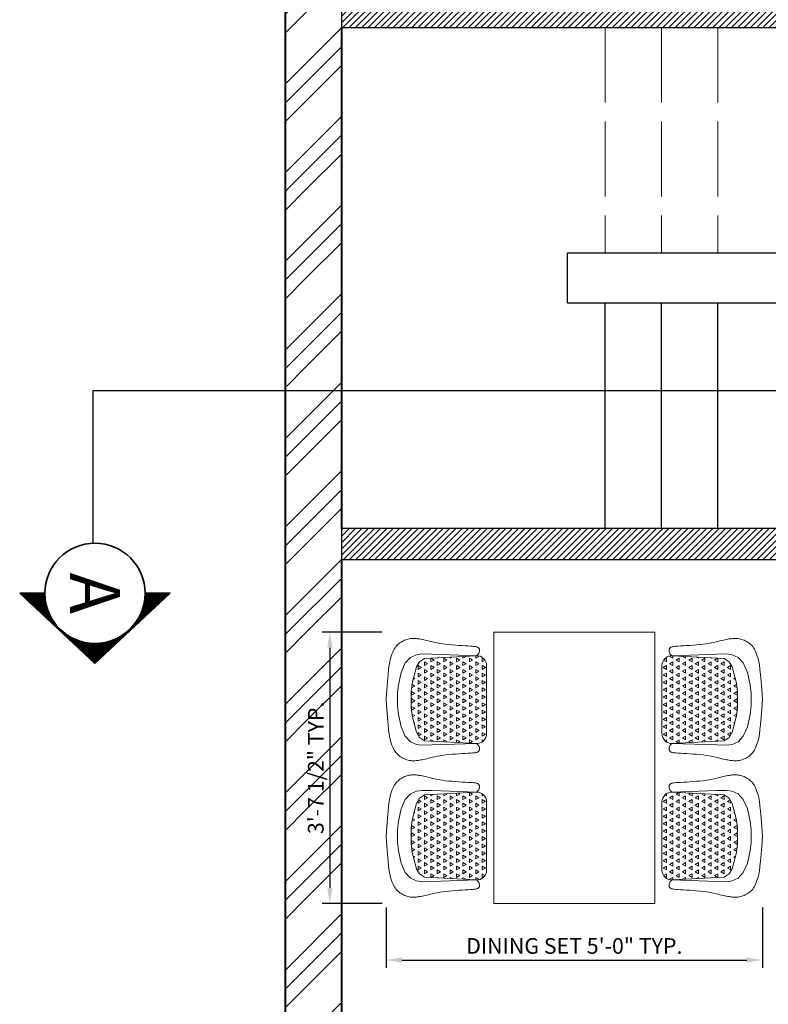
# Model space of a CAD drawing. Units: inches. Extents: x 2443635 to 2446153, y 1826255 to 1827341.
# Tile 2 of 16: x 2443665 to 2443784, y 1826991 to 1827149. Entities that reach past the tile are written whole.
import ezdxf
from ezdxf.enums import TextEntityAlignment as Align

# ---------------------------------------------------------------- set-up
doc = ezdxf.new("R2010")
doc.units = ezdxf.units.IN
doc.linetypes.add('ACAD_ISO02W100', pattern=[15, 12, -3])
for name, color, linetype, lineweight in [('A-ANNO-SYMB', 4, 'Continuous', 25), ('A-DIMS', 1, 'Continuous', 18), ('A-FURN', 6, 'Continuous', 18), ('A-SECT', 7, 'Continuous', 35), ('A-STAIR', 7, 'Continuous', 25), ('A-STAIR-OVHD', 7, 'ACAD_ISO02W100', 18), ('A-WALL-EXT', 7, 'Continuous', 40), ('A-WALL-INT', 9, 'Continuous', 30), ('A-WALL-PATT', 8, 'Continuous', 13)]:
    doc.layers.add(name, color=color, linetype=linetype, lineweight=lineweight)
doc.styles.add('KH-TRUC', font='txt', dxfattribs={"height": 200})
doc.styles.get("Standard").update_dxf_attribs({"font": 'arial.ttf'})
doc.dimstyles.new('ISO-25', dxfattribs={"dimtxt": 2.5, "dimasz": 2.5, "dimexe": 1.25, "dimexo": 0.625, "dimtad": 1, "dimlunit": 4, "dimtxsty": 'Standard', "dimcen": 2.5, "dimadec": 0, "dimazin": 0, "dimtfac": 1, "dimtmove": 0, "dimatfit": 3, "dimfxl": 1, "dimarcsym": 0})

# ---------------------------------------------------------------- blocks, each defined once
blk = doc.blocks.new('*X10')
at = {"color": 0}
for p, q in [((152.437, 136.074), (152.218, 136.074)), ((152.347, 136.232), (152.437, 136.074)), ((152.625, 135.749), (152.437, 135.425)), ((152.625, 135.749), (152.812, 135.425)), ((153, 136.399), (152.812, 136.074)), ((153.187, 136.074), (152.812, 136.074)), ((153, 136.399), (153.187, 136.074)), ((153.375, 135.749), (153.187, 135.425)), ((153.375, 135.749), (153.562, 135.425)), ((153.75, 136.399), (153.562, 136.074)), ((153.937, 136.074), (153.562, 136.074)), ((153.75, 136.399), (153.937, 136.074)), ((154.125, 135.749), (153.937, 135.425)), ((154.125, 135.749), (154.312, 135.425)), ((154.5, 136.399), (154.312, 136.074)), ((154.687, 136.074), (154.312, 136.074)), ((154.5, 136.399), (154.687, 136.074)), ((154.875, 135.749), (154.687, 135.425)), ((154.875, 135.749), (155.062, 135.425)), ((155.25, 136.399), (155.062, 136.074)), ((155.437, 136.074), (155.062, 136.074)), ((155.25, 136.399), (155.437, 136.074)), ((155.625, 135.749), (155.437, 135.425)), ((155.625, 135.749), (155.812, 135.425)), ((156, 136.399), (155.812, 136.074)), ((156.187, 136.074), (155.812, 136.074)), ((156, 136.399), (156.187, 136.074)), ((156.375, 135.749), (156.187, 135.425)), ((156.375, 135.749), (156.562, 135.425)), ((156.75, 136.399), (156.562, 136.074)), ((156.937, 136.074), (156.562, 136.074)), ((156.75, 136.399), (156.937, 136.074)), ((157.125, 135.749), (156.937, 135.425)), ((157.125, 135.749), (157.312, 135.425)), ((157.5, 136.399), (157.312, 136.074)), ((157.687, 136.074), (157.312, 136.074)), ((157.5, 136.399), (157.687, 136.074)), ((157.875, 135.749), (157.687, 135.425)), ((157.875, 135.749), (158.062, 135.425)), ((158.25, 136.399), (158.062, 136.074)), ((158.437, 136.074), (158.062, 136.074)), ((158.25, 136.399), (158.437, 136.074)), ((158.625, 135.749), (158.437, 135.425)), ((158.625, 135.749), (158.812, 135.425)), ((159, 136.399), (158.812, 136.074)), ((159.187, 136.074), (158.812, 136.074)), ((159, 136.399), (159.187, 136.074)), ((159.375, 135.749), (159.187, 135.425)), ((159.375, 135.749), (159.562, 135.425)), ((159.75, 136.399), (159.562, 136.074)), ((159.937, 136.074), (159.562, 136.074)), ((159.75, 136.399), (159.937, 136.074)), ((160.125, 135.749), (159.937, 135.425)), ((160.125, 135.749), (160.312, 135.425)), ((160.482, 136.367), (160.312, 136.074)), ((160.687, 136.074), (160.312, 136.074)), ((160.542, 136.326), (160.687, 136.074)), ((160.875, 135.749), (160.687, 135.425)), ((160.875, 135.749), (160.938, 135.64)), ((152.056, 135.437), (152.062, 135.425)), ((152.062, 135.425), (152.056, 135.425)), ((152.25, 135.1), (152.089, 134.82)), ((152.437, 134.775), (152.091, 134.775)), ((152.25, 135.1), (152.437, 134.775)), ((152.812, 135.425), (152.437, 135.425)), ((153, 135.1), (152.812, 134.775)), ((153.187, 134.775), (152.812, 134.775)), ((153, 135.1), (153.187, 134.775)), ((153.562, 135.425), (153.187, 135.425)), ((153.75, 135.1), (153.562, 134.775)), ((153.937, 134.775), (153.562, 134.775)), ((153.75, 135.1), (153.937, 134.775)), ((154.312, 135.425), (153.937, 135.425)), ((154.5, 135.1), (154.312, 134.775)), ((154.687, 134.775), (154.312, 134.775)), ((154.5, 135.1), (154.687, 134.775)), ((155.062, 135.425), (154.687, 135.425)), ((155.25, 135.1), (155.062, 134.775)), ((155.437, 134.775), (155.062, 134.775)), ((155.25, 135.1), (155.437, 134.775)), ((155.812, 135.425), (155.437, 135.425)), ((156, 135.1), (155.812, 134.775)), ((156.187, 134.775), (155.812, 134.775)), ((156, 135.1), (156.187, 134.775)), ((156.562, 135.425), (156.187, 135.425)), ((156.75, 135.1), (156.562, 134.775)), ((156.937, 134.775), (156.562, 134.775)), ((156.75, 135.1), (156.937, 134.775)), ((157.312, 135.425), (156.937, 135.425)), ((157.5, 135.1), (157.312, 134.775)), ((157.687, 134.775), (157.312, 134.775)), ((157.5, 135.1), (157.687, 134.775)), ((158.062, 135.425), (157.687, 135.425)), ((158.25, 135.1), (158.062, 134.775)), ((158.437, 134.775), (158.062, 134.775)), ((158.25, 135.1), (158.437, 134.775)), ((158.812, 135.425), (158.437, 135.425)), ((159, 135.1), (158.812, 134.775)), ((159.187, 134.775), (158.812, 134.775)), ((159, 135.1), (159.187, 134.775)), ((159.562, 135.425), (159.187, 135.425)), ((159.75, 135.1), (159.562, 134.775)), ((159.937, 134.775), (159.562, 134.775)), ((159.75, 135.1), (159.937, 134.775)), ((160.312, 135.425), (159.937, 135.425)), ((160.5, 135.1), (160.312, 134.775)), ((160.687, 134.775), (160.312, 134.775)), ((160.5, 135.1), (160.687, 134.775)), ((160.941, 135.425), (160.687, 135.425)), ((152.25, 133.801), (152.152, 133.631)), ((152.25, 133.801), (152.437, 133.476)), ((152.625, 134.45), (152.437, 134.126)), ((152.812, 134.126), (152.437, 134.126)), ((152.625, 134.45), (152.812, 134.126)), ((153, 133.801), (152.812, 133.476)), ((153, 133.801), (153.187, 133.476)), ((153.375, 134.45), (153.187, 134.126)), ((153.562, 134.126), (153.187, 134.126)), ((153.375, 134.45), (153.562, 134.126)), ((153.75, 133.801), (153.562, 133.476)), ((153.75, 133.801), (153.937, 133.476)), ((154.125, 134.45), (153.937, 134.126)), ((154.312, 134.126), (153.937, 134.126)), ((154.125, 134.45), (154.312, 134.126)), ((154.5, 133.801), (154.312, 133.476)), ((154.5, 133.801), (154.687, 133.476)), ((154.875, 134.45), (154.687, 134.126)), ((155.062, 134.126), (154.687, 134.126)), ((154.875, 134.45), (155.062, 134.126)), ((155.25, 133.801), (155.062, 133.476)), ((155.25, 133.801), (155.437, 133.476)), ((155.625, 134.45), (155.437, 134.126)), ((155.812, 134.126), (155.437, 134.126)), ((155.625, 134.45), (155.812, 134.126)), ((156, 133.801), (155.812, 133.476)), ((156, 133.801), (156.187, 133.476)), ((156.375, 134.45), (156.187, 134.126)), ((156.562, 134.126), (156.187, 134.126)), ((156.375, 134.45), (156.562, 134.126)), ((156.75, 133.801), (156.562, 133.476)), ((156.75, 133.801), (156.937, 133.476)), ((157.125, 134.45), (156.937, 134.126)), ((157.312, 134.126), (156.937, 134.126)), ((157.125, 134.45), (157.312, 134.126)), ((157.5, 133.801), (157.312, 133.476)), ((157.5, 133.801), (157.687, 133.476)), ((157.875, 134.45), (157.687, 134.126)), ((158.062, 134.126), (157.687, 134.126)), ((157.875, 134.45), (158.062, 134.126)), ((158.25, 133.801), (158.062, 133.476)), ((158.25, 133.801), (158.437, 133.476)), ((158.625, 134.45), (158.437, 134.126)), ((158.812, 134.126), (158.437, 134.126)), ((158.625, 134.45), (158.812, 134.126)), ((159, 133.801), (158.812, 133.476)), ((159, 133.801), (159.187, 133.476)), ((159.375, 134.45), (159.187, 134.126)), ((159.562, 134.126), (159.187, 134.126)), ((159.375, 134.45), (159.562, 134.126)), ((159.75, 133.801), (159.562, 133.476)), ((159.75, 133.801), (159.937, 133.476)), ((160.125, 134.45), (159.937, 134.126)), ((160.312, 134.126), (159.937, 134.126)), ((160.125, 134.45), (160.312, 134.126)), ((160.5, 133.801), (160.312, 133.476)), ((160.5, 133.801), (160.687, 133.476)), ((160.875, 134.45), (160.687, 134.126)), ((160.872, 134.126), (160.687, 134.126)), ((160.875, 134.45), (160.888, 134.428)), ((152.437, 133.476), (152.16, 133.476)), ((152.625, 133.151), (152.437, 132.827)), ((152.812, 132.827), (152.437, 132.827)), ((152.625, 133.151), (152.812, 132.827)), ((153.187, 133.476), (152.812, 133.476)), ((153.375, 133.151), (153.187, 132.827)), ((153.562, 132.827), (153.187, 132.827)), ((153.375, 133.151), (153.562, 132.827)), ((153.937, 133.476), (153.562, 133.476)), ((154.125, 133.151), (153.937, 132.827)), ((154.312, 132.827), (153.937, 132.827)), ((154.125, 133.151), (154.312, 132.827)), ((154.687, 133.476), (154.312, 133.476)), ((154.875, 133.151), (154.687, 132.827)), ((155.062, 132.827), (154.687, 132.827)), ((154.875, 133.151), (155.062, 132.827)), ((155.437, 133.476), (155.062, 133.476)), ((155.625, 133.151), (155.437, 132.827)), ((155.812, 132.827), (155.437, 132.827)), ((155.625, 133.151), (155.812, 132.827)), ((156.187, 133.476), (155.812, 133.476)), ((156.375, 133.151), (156.187, 132.827)), ((156.562, 132.827), (156.187, 132.827)), ((156.375, 133.151), (156.562, 132.827)), ((156.937, 133.476), (156.562, 133.476)), ((157.125, 133.151), (156.937, 132.827)), ((157.312, 132.827), (156.937, 132.827)), ((157.125, 133.151), (157.312, 132.827)), ((157.687, 133.476), (157.312, 133.476)), ((157.875, 133.151), (157.687, 132.827)), ((158.062, 132.827), (157.687, 132.827)), ((157.875, 133.151), (158.062, 132.827)), ((158.437, 133.476), (158.062, 133.476)), ((158.625, 133.151), (158.437, 132.827)), ((158.812, 132.827), (158.437, 132.827)), ((158.625, 133.151), (158.812, 132.827)), ((159.187, 133.476), (158.812, 133.476)), ((159.375, 133.151), (159.187, 132.827)), ((159.562, 132.827), (159.187, 132.827)), ((159.375, 133.151), (159.562, 132.827)), ((159.937, 133.476), (159.562, 133.476)), ((160.125, 133.151), (159.937, 132.827)), ((160.312, 132.827), (159.937, 132.827)), ((160.125, 133.151), (160.312, 132.827)), ((160.687, 133.476), (160.312, 133.476)), ((160.814, 133.046), (160.687, 132.827)), ((160.803, 132.827), (160.687, 132.827)), ((152.25, 132.502), (152.216, 132.442)), ((152.437, 132.177), (152.23, 132.177)), ((152.25, 132.502), (152.437, 132.177)), ((152.625, 131.852), (152.437, 131.528)), ((152.625, 131.852), (152.812, 131.528)), ((153, 132.502), (152.812, 132.177)), ((153.187, 132.177), (152.812, 132.177)), ((153, 132.502), (153.187, 132.177)), ((153.375, 131.852), (153.187, 131.528)), ((153.375, 131.852), (153.562, 131.528)), ((153.75, 132.502), (153.562, 132.177)), ((153.937, 132.177), (153.562, 132.177)), ((153.75, 132.502), (153.937, 132.177)), ((154.125, 131.852), (153.937, 131.528)), ((154.125, 131.852), (154.312, 131.528)), ((154.5, 132.502), (154.312, 132.177)), ((154.687, 132.177), (154.312, 132.177)), ((154.5, 132.502), (154.687, 132.177)), ((154.875, 131.852), (154.687, 131.528)), ((154.875, 131.852), (155.062, 131.528)), ((155.25, 132.502), (155.062, 132.177)), ((155.437, 132.177), (155.062, 132.177)), ((155.25, 132.502), (155.437, 132.177)), ((155.625, 131.852), (155.437, 131.528)), ((155.625, 131.852), (155.812, 131.528)), ((156, 132.502), (155.812, 132.177)), ((156.187, 132.177), (155.812, 132.177)), ((156, 132.502), (156.187, 132.177)), ((156.375, 131.852), (156.187, 131.528)), ((156.375, 131.852), (156.562, 131.528)), ((156.75, 132.502), (156.562, 132.177)), ((156.937, 132.177), (156.562, 132.177)), ((156.75, 132.502), (156.937, 132.177)), ((157.125, 131.852), (156.937, 131.528)), ((157.125, 131.852), (157.312, 131.528)), ((157.5, 132.502), (157.312, 132.177)), ((157.687, 132.177), (157.312, 132.177)), ((157.5, 132.502), (157.687, 132.177)), ((157.875, 131.852), (157.687, 131.528)), ((157.875, 131.852), (158.062, 131.528)), ((158.25, 132.502), (158.062, 132.177)), ((158.437, 132.177), (158.062, 132.177)), ((158.25, 132.502), (158.437, 132.177)), ((158.625, 131.852), (158.437, 131.528)), ((158.625, 131.852), (158.812, 131.528)), ((159, 132.502), (158.812, 132.177)), ((159.187, 132.177), (158.812, 132.177)), ((159, 132.502), (159.187, 132.177)), ((159.375, 131.852), (159.187, 131.528)), ((159.375, 131.852), (159.562, 131.528)), ((159.75, 132.502), (159.562, 132.177)), ((159.937, 132.177), (159.562, 132.177)), ((159.75, 132.502), (159.937, 132.177)), ((160.125, 131.852), (159.937, 131.528)), ((160.125, 131.852), (160.312, 131.528)), ((160.5, 132.502), (160.312, 132.177)), ((160.687, 132.177), (160.312, 132.177)), ((160.5, 132.502), (160.687, 132.177)), ((160.738, 131.615), (160.687, 131.528)), ((152.285, 131.142), (152.437, 130.878)), ((152.437, 130.878), (152.299, 130.878)), ((152.812, 131.528), (152.437, 131.528)), ((153, 131.203), (152.812, 130.878)), ((153.187, 130.878), (152.812, 130.878)), ((153, 131.203), (153.187, 130.878)), ((153.562, 131.528), (153.187, 131.528)), ((153.75, 131.203), (153.562, 130.878)), ((153.937, 130.878), (153.562, 130.878)), ((153.75, 131.203), (153.937, 130.878)), ((154.312, 131.528), (153.937, 131.528)), ((154.5, 131.203), (154.312, 130.878)), ((154.687, 130.878), (154.312, 130.878)), ((154.5, 131.203), (154.687, 130.878)), ((155.062, 131.528), (154.687, 131.528)), ((155.25, 131.203), (155.062, 130.878)), ((155.437, 130.878), (155.062, 130.878)), ((155.25, 131.203), (155.437, 130.878)), ((155.812, 131.528), (155.437, 131.528)), ((156, 131.203), (155.812, 130.878)), ((156.187, 130.878), (155.812, 130.878)), ((156, 131.203), (156.187, 130.878)), ((156.562, 131.528), (156.187, 131.528)), ((156.75, 131.203), (156.562, 130.878)), ((156.937, 130.878), (156.562, 130.878)), ((156.75, 131.203), (156.937, 130.878)), ((157.312, 131.528), (156.937, 131.528)), ((157.5, 131.203), (157.312, 130.878)), ((157.687, 130.878), (157.312, 130.878)), ((157.5, 131.203), (157.687, 130.878)), ((158.062, 131.528), (157.687, 131.528)), ((158.25, 131.203), (158.062, 130.878)), ((158.437, 130.878), (158.062, 130.878)), ((158.25, 131.203), (158.437, 130.878)), ((158.812, 131.528), (158.437, 131.528)), ((159, 131.203), (158.812, 130.878)), ((159.187, 130.878), (158.812, 130.878)), ((159, 131.203), (159.187, 130.878)), ((159.562, 131.528), (159.187, 131.528)), ((159.75, 131.203), (159.562, 130.878)), ((159.937, 130.878), (159.562, 130.878)), ((159.75, 131.203), (159.937, 130.878)), ((160.312, 131.528), (159.937, 131.528)), ((160.5, 131.203), (160.312, 130.878)), ((160.687, 130.878), (160.312, 130.878)), ((160.5, 131.203), (160.687, 130.878)), ((160.733, 131.528), (160.687, 131.528)), ((152.625, 130.553), (152.437, 130.229)), ((152.812, 130.229), (152.437, 130.229)), ((152.625, 130.553), (152.812, 130.229)), ((153, 129.904), (152.842, 129.63)), ((153, 129.904), (153.187, 129.579)), ((153.375, 130.553), (153.187, 130.229)), ((153.562, 130.229), (153.187, 130.229)), ((153.375, 130.553), (153.562, 130.229)), ((153.75, 129.904), (153.562, 129.579)), ((153.75, 129.904), (153.937, 129.579)), ((154.125, 130.553), (153.937, 130.229)), ((154.312, 130.229), (153.937, 130.229)), ((154.125, 130.553), (154.312, 130.229)), ((154.5, 129.904), (154.312, 129.579)), ((154.5, 129.904), (154.687, 129.579)), ((154.875, 130.553), (154.687, 130.229)), ((155.062, 130.229), (154.687, 130.229)), ((154.875, 130.553), (155.062, 130.229)), ((155.25, 129.904), (155.062, 129.579)), ((155.25, 129.904), (155.437, 129.579)), ((155.625, 130.553), (155.437, 130.229)), ((155.812, 130.229), (155.437, 130.229)), ((155.625, 130.553), (155.812, 130.229)), ((156, 129.904), (155.812, 129.579)), ((156, 129.904), (156.187, 129.579)), ((156.375, 130.553), (156.187, 130.229)), ((156.562, 130.229), (156.187, 130.229)), ((156.375, 130.553), (156.562, 130.229)), ((156.75, 129.904), (156.562, 129.579)), ((156.75, 129.904), (156.937, 129.579)), ((157.125, 130.553), (156.937, 130.229)), ((157.312, 130.229), (156.937, 130.229)), ((157.125, 130.553), (157.312, 130.229)), ((157.5, 129.904), (157.312, 129.579)), ((157.5, 129.904), (157.687, 129.579)), ((157.875, 130.553), (157.687, 130.229)), ((158.062, 130.229), (157.687, 130.229)), ((157.875, 130.553), (158.062, 130.229)), ((158.25, 129.904), (158.062, 129.579)), ((158.25, 129.904), (158.437, 129.579)), ((158.625, 130.553), (158.437, 130.229)), ((158.812, 130.229), (158.437, 130.229)), ((158.625, 130.553), (158.812, 130.229)), ((159, 129.904), (158.812, 129.579)), ((159, 129.904), (159.187, 129.579)), ((159.375, 130.553), (159.187, 130.229)), ((159.562, 130.229), (159.187, 130.229)), ((159.375, 130.553), (159.562, 130.229)), ((159.75, 129.904), (159.562, 129.579)), ((159.75, 129.904), (159.937, 129.579)), ((160.125, 130.553), (159.937, 130.229)), ((160.312, 130.229), (159.937, 130.229)), ((160.125, 130.553), (160.312, 130.229)), ((153.187, 129.579), (152.929, 129.579)), ((153.937, 129.579), (153.562, 129.579)), ((154.125, 129.254), (154.089, 129.192)), ((154.125, 129.254), (154.174, 129.17)), ((154.687, 129.579), (154.312, 129.579)), ((154.875, 129.254), (154.741, 129.023)), ((154.875, 129.254), (155.04, 128.968)), ((155.437, 129.579), (155.062, 129.579)), ((155.625, 129.254), (155.437, 128.93)), ((155.812, 128.93), (155.437, 128.93)), ((155.625, 129.254), (155.812, 128.93)), ((156.187, 129.579), (155.812, 129.579)), ((156.375, 129.254), (156.187, 128.93)), ((156.562, 128.93), (156.187, 128.93)), ((156.375, 129.254), (156.562, 128.93)), ((156.937, 129.579), (156.562, 129.579)), ((157.125, 129.254), (156.937, 128.93)), ((157.312, 128.93), (156.937, 128.93)), ((157.125, 129.254), (157.312, 128.93)), ((157.687, 129.579), (157.312, 129.579)), ((157.875, 129.254), (157.688, 128.93)), ((157.875, 129.254), (158.034, 128.979)), ((158.437, 129.579), (158.062, 129.579)), ((158.625, 129.254), (158.533, 129.095)), ((158.625, 129.254), (158.693, 129.136)), ((159.187, 129.579), (158.812, 129.579)), ((159.937, 129.579), (159.562, 129.579))]:
    blk.add_line(p, q, dxfattribs=at)
blk = doc.blocks.new('A$C36D1434F')
at = {"layer": 'A-FURN'}
for p, q in [((0, 534.2), (0, 1334.2)), ((0, 1334.2), (1350, 1334.2)), ((1350, 1334.2), (1350, 534.2)), ((1350, 534.2), (0, 534.2))]:
    blk.add_line(p, q, dxfattribs=at)
for points in [[(117.6, 1418.8), (113.4, 1414.5), (109.3, 1411.1), (105.6, 1408.5), (102.1, 1406.7), (98.8, 1405.6), (95.7, 1404.9), (92.9, 1404.7), (90.4, 1404.8), (88.1, 1405.1), (85.9, 1405.5), (84, 1406.2), (82.3, 1407), (80.7, 1408), (79.3, 1409.1), (78, 1410.4), (76.9, 1411.8), (75.8, 1413.4), (74.8, 1415.4), (73.8, 1418.1), (73, 1421.7), (72.1, 1426.5), (71.4, 1432.7), (70.6, 1440.7), (69.8, 1450.6), (69.1, 1462.6), (68.3, 1476.5), (67.4, 1491.7), (66.5, 1507.9), (65.3, 1524.7), (64.1, 1541.5), (62.6, 1558.1), (60.8, 1574), (58.8, 1588.9), (56.6, 1602.7), (54.2, 1615.4), (51.7, 1627.3), (49.2, 1638.3), (46.8, 1648.5), (44.5, 1657.9), (42.3, 1666.7), (40.3, 1674.8), (38.6, 1682.4), (37.1, 1689.6), (35.8, 1696.3), (34.7, 1702.7), (33.8, 1708.8), (33.1, 1714.7), (32.5, 1720.5), (32.1, 1726.2), (31.9, 1731.8), (32, 1737.5), (32.3, 1743.1), (32.8, 1748.7), (33.7, 1754.3), (34.9, 1760), (36.5, 1765.8), (38.5, 1771.7), (40.9, 1777.6), (43.6, 1783.5), (46.7, 1789.3), (50.2, 1795.1), (54, 1800.6), (58.1, 1806), (62.6, 1811.1), (67.4, 1816), (72.6, 1820.5), (78.3, 1824.8), (84.8, 1828.9), (92, 1832.8), (100.2, 1836.5), (109.5, 1840.1), (119.9, 1843.5), (131.9, 1846.9), (146.1, 1850.2), (163.5, 1853.5), (185.3, 1856.6), (212.3, 1859.7), (245.5, 1862.7), (285.9, 1865.6), (334.5, 1868.4)], [(554.3, 1418.8), (558.6, 1414.5), (562.6, 1411.1), (566.3, 1408.5), (569.9, 1406.7), (573.1, 1405.6), (576.2, 1404.9), (579, 1404.7), (581.5, 1404.8), (583.9, 1405.1), (586, 1405.5), (587.9, 1406.2), (589.6, 1407), (591.2, 1408), (592.6, 1409.1), (593.9, 1410.4), (595.1, 1411.8), (596.2, 1413.4), (597.2, 1415.4), (598.1, 1418.1), (599, 1421.7), (599.8, 1426.5), (600.6, 1432.7), (601.3, 1440.7), (602.1, 1450.6), (602.8, 1462.6), (603.6, 1476.5), (604.5, 1491.7), (605.5, 1507.9), (606.6, 1524.7), (607.9, 1541.5), (609.4, 1558.1), (611.1, 1574), (613.1, 1588.9), (615.3, 1602.7), (617.7, 1615.4), (620.2, 1627.3), (622.7, 1638.3), (625.1, 1648.5), (627.5, 1657.9), (629.6, 1666.7), (631.6, 1674.8), (633.3, 1682.4), (634.8, 1689.6), (636.1, 1696.3), (637.2, 1702.7), (638.1, 1708.8), (638.9, 1714.7), (639.4, 1720.5), (639.8, 1726.2), (640, 1731.8), (640, 1737.5), (639.7, 1743.1), (639.1, 1748.7), (638.2, 1754.3), (637, 1760), (635.4, 1765.8), (633.4, 1771.7), (631.1, 1777.6), (628.3, 1783.5), (625.2, 1789.3), (621.7, 1795.1), (617.9, 1800.6), (613.8, 1806), (609.4, 1811.1), (604.6, 1816), (599.4, 1820.5), (593.6, 1824.8), (587.1, 1828.9), (579.9, 1832.8), (571.7, 1836.5), (562.4, 1840.1), (552, 1843.5), (540.1, 1846.9), (525.8, 1850.2), (508.2, 1853.5), (486.3, 1856.6), (458.9, 1859.7), (425.2, 1862.7), (384.1, 1865.6), (334.5, 1868.4)], [(795.7, 1418.8), (791.4, 1414.5), (787.4, 1411.1), (783.7, 1408.5), (780.1, 1406.7), (776.9, 1405.6), (773.8, 1404.9), (771, 1404.7), (768.5, 1404.8), (766.1, 1405.1), (764, 1405.5), (762.1, 1406.2), (760.4, 1407), (758.8, 1408), (757.4, 1409.1), (756.1, 1410.4), (754.9, 1411.8), (753.8, 1413.4), (752.8, 1415.4), (751.9, 1418.1), (751, 1421.7), (750.2, 1426.5), (749.4, 1432.7), (748.7, 1440.7), (747.9, 1450.6), (747.2, 1462.6), (746.4, 1476.5), (745.5, 1491.7), (744.5, 1507.9), (743.4, 1524.7), (742.1, 1541.5), (740.6, 1558.1), (738.9, 1574), (736.9, 1588.9), (734.7, 1602.7), (732.3, 1615.4), (729.8, 1627.3), (727.3, 1638.3), (724.9, 1648.5), (722.5, 1657.9), (720.4, 1666.7), (718.4, 1674.8), (716.7, 1682.4), (715.2, 1689.6), (713.9, 1696.3), (712.8, 1702.7), (711.9, 1708.8), (711.1, 1714.7), (710.6, 1720.5), (710.2, 1726.2), (710, 1731.8), (710, 1737.5), (710.3, 1743.1), (710.9, 1748.7), (711.8, 1754.3), (713, 1760), (714.6, 1765.8), (716.6, 1771.7), (718.9, 1777.6), (721.7, 1783.5), (724.8, 1789.3), (728.3, 1795.1), (732.1, 1800.6), (736.2, 1806), (740.6, 1811.1), (745.4, 1816), (750.6, 1820.5), (756.4, 1824.8), (762.9, 1828.9), (770.1, 1832.8), (778.3, 1836.5), (787.6, 1840.1), (798, 1843.5), (809.9, 1846.9), (824.2, 1850.2), (841.8, 1853.5), (863.7, 1856.6), (891.1, 1859.7), (924.8, 1862.7), (965.9, 1865.6), (1015.5, 1868.4)], [(1232.4, 1418.8), (1236.6, 1414.5), (1240.7, 1411.1), (1244.4, 1408.5), (1247.9, 1406.7), (1251.2, 1405.6), (1254.3, 1404.9), (1257.1, 1404.7), (1259.6, 1404.8), (1261.9, 1405.1), (1264.1, 1405.5), (1266, 1406.2), (1267.7, 1407), (1269.3, 1408), (1270.7, 1409.1), (1272, 1410.4), (1273.1, 1411.8), (1274.2, 1413.4), (1275.2, 1415.4), (1276.2, 1418.1), (1277, 1421.7), (1277.9, 1426.5), (1278.6, 1432.7), (1279.4, 1440.7), (1280.2, 1450.6), (1280.9, 1462.6), (1281.7, 1476.5), (1282.6, 1491.7), (1283.5, 1507.9), (1284.7, 1524.7), (1285.9, 1541.5), (1287.4, 1558.1), (1289.2, 1574), (1291.2, 1588.9), (1293.4, 1602.7), (1295.8, 1615.4), (1298.3, 1627.3), (1300.8, 1638.3), (1303.2, 1648.5), (1305.5, 1657.9), (1307.7, 1666.7), (1309.7, 1674.8), (1311.4, 1682.4), (1312.9, 1689.6), (1314.2, 1696.3), (1315.3, 1702.7), (1316.2, 1708.8), (1316.9, 1714.7), (1317.5, 1720.5), (1317.9, 1726.2), (1318.1, 1731.8), (1318, 1737.5), (1317.7, 1743.1), (1317.2, 1748.7), (1316.3, 1754.3), (1315.1, 1760), (1313.5, 1765.8), (1311.5, 1771.7), (1309.1, 1777.6), (1306.4, 1783.5), (1303.3, 1789.3), (1299.8, 1795.1), (1296, 1800.6), (1291.9, 1806), (1287.4, 1811.1), (1282.6, 1816), (1277.4, 1820.5), (1271.7, 1824.8), (1265.2, 1828.9), (1258, 1832.8), (1249.8, 1836.5), (1240.5, 1840.1), (1230.1, 1843.5), (1218.1, 1846.9), (1203.9, 1850.2), (1186.5, 1853.5), (1164.7, 1856.6), (1137.7, 1859.7), (1104.5, 1862.7), (1064.1, 1865.6), (1015.5, 1868.4)], [(117.6, 1418.8), (110.4, 1641.6), (108.9, 1691.2), (113.4, 1718.2), (127, 1748.3), (154, 1773.8), (200.6, 1794.9), (262.2, 1808.4), (304.3, 1812.9), (337.4, 1812.9)], [(554.3, 1418.8), (561.5, 1641.6), (563, 1691.2), (558.5, 1718.2), (545, 1748.3), (517.9, 1773.8), (471.3, 1794.9), (409.7, 1808.4), (367.6, 1812.9), (334.5, 1812.9)], [(795.7, 1418.8), (788.5, 1641.6), (787, 1691.2), (791.5, 1718.2), (805, 1748.3), (832.1, 1773.8), (878.7, 1794.9), (940.3, 1808.4), (982.4, 1812.9), (1015.5, 1812.9)], [(1232.4, 1418.8), (1239.6, 1641.6), (1241.1, 1691.2), (1236.6, 1718.2), (1223, 1748.3), (1196, 1773.8), (1149.4, 1794.9), (1087.8, 1808.4), (1045.7, 1812.9), (1012.6, 1812.9)], [(117.6, 449.6), (113.4, 453.9), (109.3, 457.3), (105.6, 459.9), (102.1, 461.7), (98.8, 462.8), (95.7, 463.5), (92.9, 463.7), (90.4, 463.6), (88.1, 463.3), (85.9, 462.9), (84, 462.2), (82.3, 461.4), (80.7, 460.4), (79.3, 459.3), (78, 458), (76.9, 456.6), (75.8, 455), (74.8, 453), (73.8, 450.3), (73, 446.7), (72.1, 441.9), (71.4, 435.6), (70.6, 427.7), (69.8, 417.8), (69.1, 405.8), (68.3, 391.9), (67.4, 376.7), (66.5, 360.5), (65.3, 343.7), (64.1, 326.9), (62.6, 310.3), (60.8, 294.4), (58.8, 279.5), (56.6, 265.7), (54.2, 252.9), (51.7, 241.1), (49.2, 230.1), (46.8, 219.9), (44.5, 210.5), (42.3, 201.7), (40.3, 193.6), (38.6, 186), (37.1, 178.8), (35.8, 172.1), (34.7, 165.7), (33.8, 159.6), (33.1, 153.7), (32.5, 147.9), (32.1, 142.2), (31.9, 136.6), (32, 130.9), (32.3, 125.3), (32.8, 119.7), (33.7, 114.1), (34.9, 108.4), (36.5, 102.6), (38.5, 96.7), (40.9, 90.8), (43.6, 84.9), (46.7, 79.1), (50.2, 73.3), (54, 67.8), (58.1, 62.4), (62.6, 57.3), (67.4, 52.4), (72.6, 47.9), (78.3, 43.6), (84.8, 39.5), (92, 35.6), (100.2, 31.9), (109.5, 28.3), (119.9, 24.8), (131.9, 21.5), (146.1, 18.2), (163.5, 14.9), (185.3, 11.8), (212.3, 8.7), (245.5, 5.7), (285.9, 2.8), (334.5, 0)], [(117.6, 449.6), (110.4, 226.8), (108.9, 177.2), (113.4, 150.2), (127, 120.1), (154, 94.6), (200.6, 73.5), (262.2, 60), (304.3, 55.5), (337.4, 55.5)], [(554.3, 449.6), (558.6, 453.9), (562.6, 457.3), (566.3, 459.9), (569.9, 461.7), (573.1, 462.8), (576.2, 463.5), (579, 463.7), (581.5, 463.6), (583.9, 463.3), (586, 462.9), (587.9, 462.2), (589.6, 461.4), (591.2, 460.4), (592.6, 459.3), (593.9, 458), (595.1, 456.6), (596.2, 455), (597.2, 453), (598.1, 450.3), (599, 446.7), (599.8, 441.9), (600.6, 435.6), (601.3, 427.7), (602.1, 417.8), (602.8, 405.8), (603.6, 391.9), (604.5, 376.7), (605.5, 360.5), (606.6, 343.7), (607.9, 326.9), (609.4, 310.3), (611.1, 294.4), (613.1, 279.5), (615.3, 265.7), (617.7, 252.9), (620.2, 241.1), (622.7, 230.1), (625.1, 219.9), (627.5, 210.5), (629.6, 201.7), (631.6, 193.6), (633.3, 186), (634.8, 178.8), (636.1, 172.1), (637.2, 165.7), (638.1, 159.6), (638.9, 153.7), (639.4, 147.9), (639.8, 142.2), (640, 136.6), (640, 130.9), (639.7, 125.3), (639.1, 119.7), (638.2, 114.1), (637, 108.4), (635.4, 102.6), (633.4, 96.7), (631.1, 90.8), (628.3, 84.9), (625.2, 79.1), (621.7, 73.3), (617.9, 67.8), (613.8, 62.4), (609.4, 57.3), (604.6, 52.4), (599.4, 47.9), (593.6, 43.6), (587.1, 39.5), (579.9, 35.6), (571.7, 31.9), (562.4, 28.3), (552, 24.8), (540.1, 21.5), (525.8, 18.2), (508.2, 14.9), (486.3, 11.8), (458.9, 8.7), (425.2, 5.7), (384.1, 2.8), (334.5, 0)], [(554.3, 449.6), (561.5, 226.8), (563, 177.2), (558.5, 150.2), (545, 120.1), (517.9, 94.6), (471.3, 73.5), (409.7, 60), (367.6, 55.5), (334.5, 55.5)], [(795.7, 449.6), (791.4, 453.9), (787.4, 457.3), (783.7, 459.9), (780.1, 461.7), (776.9, 462.8), (773.8, 463.5), (771, 463.7), (768.5, 463.6), (766.1, 463.3), (764, 462.9), (762.1, 462.2), (760.4, 461.4), (758.8, 460.4), (757.4, 459.3), (756.1, 458), (754.9, 456.6), (753.8, 455), (752.8, 453), (751.9, 450.3), (751, 446.7), (750.2, 441.9), (749.4, 435.6), (748.7, 427.7), (747.9, 417.8), (747.2, 405.8), (746.4, 391.9), (745.5, 376.7), (744.5, 360.5), (743.4, 343.7), (742.1, 326.9), (740.6, 310.3), (738.9, 294.4), (736.9, 279.5), (734.7, 265.7), (732.3, 252.9), (729.8, 241.1), (727.3, 230.1), (724.9, 219.9), (722.5, 210.5), (720.4, 201.7), (718.4, 193.6), (716.7, 186), (715.2, 178.8), (713.9, 172.1), (712.8, 165.7), (711.9, 159.6), (711.1, 153.7), (710.6, 147.9), (710.2, 142.2), (710, 136.6), (710, 130.9), (710.3, 125.3), (710.9, 119.7), (711.8, 114.1), (713, 108.4), (714.6, 102.6), (716.6, 96.7), (718.9, 90.8), (721.7, 84.9), (724.8, 79.1), (728.3, 73.3), (732.1, 67.8), (736.2, 62.4), (740.6, 57.3), (745.4, 52.4), (750.6, 47.9), (756.4, 43.6), (762.9, 39.5), (770.1, 35.6), (778.3, 31.9), (787.6, 28.3), (798, 24.8), (809.9, 21.5), (824.2, 18.2), (841.8, 14.9), (863.7, 11.8), (891.1, 8.7), (924.8, 5.7), (965.9, 2.8), (1015.5, 0)], [(795.7, 449.6), (788.5, 226.8), (787, 177.2), (791.5, 150.2), (805, 120.1), (832.1, 94.6), (878.7, 73.5), (940.3, 60), (982.4, 55.5), (1015.5, 55.5)], [(1232.4, 449.6), (1239.6, 226.8), (1241.1, 177.2), (1236.6, 150.2), (1223, 120.1), (1196, 94.6), (1149.4, 73.5), (1087.8, 60), (1045.7, 55.5), (1012.6, 55.5)], [(1232.4, 449.6), (1236.6, 453.9), (1240.7, 457.3), (1244.4, 459.9), (1247.9, 461.7), (1251.2, 462.8), (1254.3, 463.5), (1257.1, 463.7), (1259.6, 463.6), (1261.9, 463.3), (1264.1, 462.9), (1266, 462.2), (1267.7, 461.4), (1269.3, 460.4), (1270.7, 459.3), (1272, 458), (1273.1, 456.6), (1274.2, 455), (1275.2, 453), (1276.2, 450.3), (1277, 446.7), (1277.9, 441.9), (1278.6, 435.6), (1279.4, 427.7), (1280.2, 417.8), (1280.9, 405.8), (1281.7, 391.9), (1282.6, 376.7), (1283.5, 360.5), (1284.7, 343.7), (1285.9, 326.9), (1287.4, 310.3), (1289.2, 294.4), (1291.2, 279.5), (1293.4, 265.7), (1295.8, 252.9), (1298.3, 241.1), (1300.8, 230.1), (1303.2, 219.9), (1305.5, 210.5), (1307.7, 201.7), (1309.7, 193.6), (1311.4, 186), (1312.9, 178.8), (1314.2, 172.1), (1315.3, 165.7), (1316.2, 159.6), (1316.9, 153.7), (1317.5, 147.9), (1317.9, 142.2), (1318.1, 136.6), (1318, 130.9), (1317.7, 125.3), (1317.2, 119.7), (1316.3, 114.1), (1315.1, 108.4), (1313.5, 102.6), (1311.5, 96.7), (1309.1, 90.8), (1306.4, 84.9), (1303.3, 79.1), (1299.8, 73.3), (1296, 67.8), (1291.9, 62.4), (1287.4, 57.3), (1282.6, 52.4), (1277.4, 47.9), (1271.7, 43.6), (1265.2, 39.5), (1258, 35.6), (1249.8, 31.9), (1240.5, 28.3), (1230.1, 24.8), (1218.1, 21.5), (1203.9, 18.2), (1186.5, 14.9), (1164.7, 11.8), (1137.7, 8.7), (1104.5, 5.7), (1064.1, 2.8), (1015.5, 0)]]:
    blk.add_lwpolyline(points, dxfattribs=at)
for points in [[(337.5, 1745.3), (375.1, 1745.3), (417.2, 1739.3), (498.4, 1718.2), (523.9, 1703.2), (540.5, 1679.2), (554.2, 1421.5, -0.429937), (505.2, 1369.7), (166.8, 1369.7, -0.429937), (117.8, 1421.5), (131.6, 1679.2), (148.1, 1703.2), (173.7, 1718.2), (254.8, 1739.3), (296.9, 1745.3), (334.5, 1745.3)], [(1012.5, 1745.3), (974.9, 1745.3), (932.8, 1739.3), (851.6, 1718.2), (826.1, 1703.2), (809.5, 1679.2), (795.8, 1421.5, 0.429937), (844.8, 1369.7), (1183.2, 1369.7, 0.429937), (1232.2, 1421.5), (1218.4, 1679.2), (1201.9, 1703.2), (1176.3, 1718.2), (1095.2, 1739.3), (1053.1, 1745.3), (1015.5, 1745.3)], [(337.5, 123.1), (375.1, 123.1), (417.2, 129.1), (498.4, 150.2), (523.9, 165.2), (540.5, 189.2), (554.2, 446.9, 0.429937), (505.2, 498.7), (166.8, 498.7, 0.429937), (117.8, 446.9), (131.6, 189.2), (148.1, 165.2), (173.7, 150.2), (254.8, 129.1), (296.9, 123.1), (334.5, 123.1)], [(1012.5, 123.1), (974.9, 123.1), (932.8, 129.1), (851.6, 150.2), (826.1, 165.2), (809.5, 189.2), (795.8, 446.9, -0.429937), (844.8, 498.7), (1183.2, 498.7, -0.429937), (1232.2, 446.9), (1218.4, 189.2), (1201.9, 165.2), (1176.3, 150.2), (1095.2, 129.1), (1053.1, 123.1), (1015.5, 123.1)]]:
    blk.add_lwpolyline(points, format="xyb", dxfattribs=at)
at = {"layer": 'A-FURN', "xscale": 49.09090909079987, "yscale": 49.09090909079987, "zscale": 49.09090909079987, "rotation": 180}
blk.add_blockref('*X10', (8018.7, 8071.8), dxfattribs=at)
at = {"layer": 'A-FURN', "extrusion": (0, 0, -1), "xscale": 49.09090909079987, "yscale": 49.09090909079987, "zscale": -49.09090909079999, "rotation": 180}
blk.add_blockref('*X10', (6668.7, 8071.8), dxfattribs=at)
at = {"layer": 'A-FURN', "extrusion": (0, 0, -1), "xscale": 49.09090909079987, "yscale": 49.09090909079987, "zscale": -49.09090909079999}
blk.add_blockref('*X10', (-8018.7, -6203.4), dxfattribs=at)
at = {"layer": 'A-FURN', "xscale": 49.09090909079987, "yscale": 49.09090909079987, "zscale": 49.09090909079987}
blk.add_blockref('*X10', (-6668.7, -6203.4), dxfattribs=at)
blk = doc.blocks.new('*X15')
at = {"color": 0}
for p, q in [((19.676, 20.472), (19.713, 20.508)), ((19.676, 20.383), (19.755, 20.462)), ((19.676, 20.295), (19.798, 20.417)), ((19.676, 20.206), (19.841, 20.371)), ((19.676, 20.118), (19.883, 20.325)), ((19.676, 20.03), (19.926, 20.279)), ((19.676, 19.941), (19.969, 20.234)), ((19.676, 19.853), (20.011, 20.188)), ((19.676, 19.764), (20.054, 20.142)), ((19.676, 19.676), (20.097, 20.097)), ((19.676, 19.588), (20.139, 20.051)), ((19.676, 19.499), (20.182, 20.005)), ((19.676, 19.411), (20.225, 19.959)), ((19.676, 19.322), (20.267, 19.914)), ((19.676, 19.234), (20.31, 19.868)), ((19.676, 19.146), (20.353, 19.822)), ((19.676, 19.057), (20.395, 19.777)), ((19.676, 18.969), (20.438, 19.731)), ((19.676, 18.881), (20.481, 19.685)), ((19.676, 18.792), (20.523, 19.639)), ((19.676, 18.704), (20.566, 19.594)), ((19.676, 18.615), (20.609, 19.548)), ((19.676, 18.527), (20.651, 19.502)), ((19.676, 18.439), (20.694, 19.457)), ((19.676, 18.35), (20.737, 19.411)), ((19.676, 18.262), (20.779, 19.365)), ((19.676, 18.173), (20.822, 19.319)), ((19.676, 18.085), (20.865, 19.274)), ((19.726, 18.047), (20.907, 19.228)), ((19.813, 18.045), (20.95, 19.182)), ((19.898, 18.042), (20.993, 19.137)), ((19.982, 18.038), (21.035, 19.091)), ((20.065, 18.032), (21.078, 19.045)), ((20.146, 18.025), (21.121, 18.999)), ((20.227, 18.017), (21.163, 18.954)), ((20.306, 18.007), (21.206, 18.908)), ((20.383, 17.997), (21.249, 18.862)), ((20.46, 17.985), (21.291, 18.816)), ((20.536, 17.973), (21.334, 18.771)), ((20.611, 17.959), (21.377, 18.725)), ((20.684, 17.944), (21.419, 18.679)), ((20.757, 17.929), (21.462, 18.634)), ((20.829, 17.912), (21.505, 18.588)), ((20.9, 17.895), (21.547, 18.542)), ((20.97, 17.877), (21.59, 18.496)), ((21.04, 17.858), (21.633, 18.451)), ((21.108, 17.838), (21.675, 18.405)), ((21.176, 17.817), (21.718, 18.359)), ((21.243, 17.795), (21.761, 18.314)), ((21.309, 17.773), (21.803, 18.268)), ((21.374, 17.75), (21.846, 18.222)), ((21.439, 17.726), (21.889, 18.176)), ((21.502, 17.702), (21.931, 18.131)), ((21.566, 17.676), (21.974, 18.085)), ((21.628, 17.65), (22.017, 18.039)), ((21.69, 17.624), (22.059, 17.994)), ((21.751, 17.596), (22.102, 17.948)), ((21.811, 17.568), (22.145, 17.902)), ((21.871, 17.54), (22.187, 17.856)), ((21.93, 17.51), (22.23, 17.811)), ((21.988, 17.48), (22.273, 17.765)), ((22.046, 17.45), (22.315, 17.719)), ((22.103, 17.419), (22.358, 17.674)), ((22.16, 17.387), (22.401, 17.628)), ((22.216, 17.354), (22.443, 17.582)), ((22.271, 17.321), (22.486, 17.536)), ((22.326, 17.287), (22.529, 17.491)), ((22.38, 17.253), (22.571, 17.445)), ((22.433, 17.218), (22.614, 17.399)), ((22.486, 17.183), (22.657, 17.353)), ((22.538, 17.147), (22.699, 17.308)), ((22.59, 17.11), (22.742, 17.262)), ((22.641, 17.073), (22.785, 17.216)), ((22.692, 17.035), (22.827, 17.171)), ((22.742, 16.997), (22.87, 17.125)), ((22.792, 16.958), (22.913, 17.079)), ((22.84, 16.918), (22.955, 17.033)), ((22.889, 16.878), (22.998, 16.988)), ((22.937, 16.838), (23.041, 16.942)), ((22.984, 16.797), (23.084, 16.896)), ((23.031, 16.755), (23.126, 16.851)), ((23.077, 16.713), (23.169, 16.805)), ((23.122, 16.67), (23.212, 16.759)), ((23.167, 16.626), (23.254, 16.713)), ((23.212, 16.583), (23.297, 16.668)), ((23.256, 16.538), (23.34, 16.622)), ((23.299, 16.493), (23.382, 16.576)), ((23.342, 16.448), (23.425, 16.531)), ((23.384, 16.401), (23.468, 16.485)), ((23.426, 16.355), (23.51, 16.439)), ((23.467, 16.307), (23.553, 16.393)), ((23.507, 16.26), (23.596, 16.348)), ((23.548, 16.211), (23.638, 16.302)), ((23.587, 16.162), (23.681, 16.256)), ((23.626, 16.113), (23.724, 16.211)), ((23.664, 16.063), (23.766, 16.165)), ((23.702, 16.012), (23.809, 16.119)), ((23.739, 15.961), (23.852, 16.073)), ((23.776, 15.909), (23.894, 16.028)), ((23.812, 15.857), (23.937, 15.982)), ((23.847, 15.804), (23.98, 15.936)), ((23.882, 15.75), (24.022, 15.891)), ((23.917, 15.696), (24.065, 15.845)), ((23.95, 15.642), (24.108, 15.799)), ((23.983, 15.586), (24.15, 15.753)), ((24.016, 15.53), (24.193, 15.708)), ((24.048, 15.474), (24.236, 15.662)), ((24.079, 15.417), (24.278, 15.616)), ((24.109, 15.359), (24.321, 15.57)), ((24.139, 15.301), (24.364, 15.525)), ((24.169, 15.242), (24.406, 15.479)), ((24.197, 15.182), (24.449, 15.433)), ((24.225, 15.121), (24.492, 15.388)), ((24.253, 15.06), (24.534, 15.342)), ((24.279, 14.999), (24.577, 15.296)), ((24.305, 14.936), (24.62, 15.25)), ((24.331, 14.873), (24.662, 15.205)), ((24.355, 14.809), (24.705, 15.159)), ((24.379, 14.745), (24.748, 15.113)), ((24.402, 14.679), (24.79, 15.068)), ((24.424, 14.613), (24.833, 15.022)), ((24.446, 14.546), (24.876, 14.976)), ((24.467, 14.479), (24.918, 14.93)), ((24.487, 14.41), (24.961, 14.885)), ((24.506, 14.341), (25.004, 14.839)), ((24.524, 14.271), (25.046, 14.793)), ((24.541, 14.2), (25.089, 14.748)), ((24.558, 14.128), (25.132, 14.702)), ((24.573, 14.055), (25.174, 14.656)), ((24.588, 13.981), (25.217, 14.61)), ((24.602, 13.907), (25.26, 14.565)), ((24.614, 13.831), (25.302, 14.519)), ((24.626, 13.754), (25.345, 14.473)), ((24.636, 13.676), (25.388, 14.428)), ((24.639, 12.442), (25.985, 13.787)), ((24.646, 13.597), (25.43, 14.382)), ((24.65, 12.541), (25.942, 13.833)), ((24.654, 13.517), (25.473, 14.336)), ((24.659, 12.638), (25.9, 13.879)), ((24.661, 13.436), (25.516, 14.29)), ((24.666, 12.734), (25.857, 13.925)), ((24.667, 13.353), (25.558, 14.245)), ((24.671, 13.269), (25.601, 14.199)), ((24.671, 12.827), (25.814, 13.97)), ((24.674, 13.184), (25.644, 14.153)), ((24.674, 12.919), (25.772, 14.016)), ((24.676, 13.097), (25.686, 14.108)), ((24.676, 13.009), (25.729, 14.062)), ((23.724, 10.112), (26.668, 13.056)), ((23.908, 10.385), (26.625, 13.102)), ((24.038, 10.603), (26.582, 13.147)), ((24.138, 10.792), (26.54, 13.193)), ((24.221, 10.962), (26.497, 13.239)), ((24.29, 11.12), (26.454, 13.285)), ((24.348, 11.267), (26.412, 13.33)), ((24.399, 11.406), (26.369, 13.376)), ((24.443, 11.538), (26.326, 13.422)), ((24.481, 11.665), (26.284, 13.467)), ((24.514, 11.787), (26.241, 13.513)), ((24.544, 11.904), (26.198, 13.559)), ((24.569, 12.018), (26.156, 13.605)), ((24.591, 12.128), (26.113, 13.65)), ((24.61, 12.235), (26.07, 13.696)), ((24.626, 12.34), (26.028, 13.742)), ((19.676, 5.976), (25.677, 11.976)), ((19.676, 5.887), (24.439, 10.651)), ((19.676, 5.799), (23.202, 9.325)), ((19.676, 6.064), (22.611, 8.999)), ((19.676, 6.153), (22.338, 8.815)), ((19.676, 6.241), (22.121, 8.686)), ((19.676, 6.329), (21.931, 8.585)), ((19.676, 6.418), (21.761, 8.503)), ((19.676, 6.506), (21.604, 8.434)), ((19.676, 6.595), (21.456, 8.375)), ((19.676, 6.683), (21.317, 8.324)), ((19.676, 6.771), (21.185, 8.28)), ((19.676, 6.86), (21.058, 8.242)), ((19.676, 6.948), (20.937, 8.209)), ((19.676, 7.036), (20.819, 8.18)), ((19.676, 7.125), (20.705, 8.154)), ((19.676, 7.213), (20.595, 8.132)), ((19.676, 7.302), (20.488, 8.114)), ((19.676, 7.39), (20.383, 8.098)), ((19.676, 7.478), (20.282, 8.084)), ((19.676, 7.567), (20.182, 8.073)), ((19.676, 7.655), (20.085, 8.064)), ((19.676, 7.744), (19.989, 8.057)), ((19.676, 7.832), (19.896, 8.052)), ((19.676, 7.92), (19.805, 8.049)), ((19.676, 8.009), (19.715, 8.047)), ((19.676, 5.711), (21.964, 7.999)), ((19.676, 5.622), (20.727, 6.673))]:
    blk.add_line(p, q, dxfattribs=at)
blk = doc.blocks.new('A$C0BB45C51')
at = {"layer": 'A-SECT'}
for p, q in [((12.857, 15), (19.857, 7.5)), ((12.857, 12.5), (12.857, 15)), ((12.857, 0), (19.857, 7.5)), ((12.857, 2.5), (12.857, 0))]:
    blk.add_line(p, q, dxfattribs=at)
blk.add_circle((12.857, 7.5), 5, dxfattribs=at)
blk.add_blockref('*X15', (-6.819, -5.547), dxfattribs=at)
at = {"layer": 'A-SECT', "style": 'KH-TRUC'}
blk.add_attdef('KH-MC', text='', height=5, dxfattribs=at).set_placement((12.857, 7.5), align=Align.MIDDLE_CENTER)
blk = doc.blocks.new('*D70')
at = {"layer": 'A-DIMS', "color": 0, "lineweight": -2, "transparency": 16777216}
for p, q in [((2443723.19, 1827006.81), (2443723.19, 1826997.19)), ((2443783.19, 1827006.81), (2443783.19, 1826997.19)), ((2443725.69, 1826998.44), (2443780.69, 1826998.44))]:
    blk.add_line(p, q, dxfattribs=at)
at = {"layer": 'A-DIMS', "color": 0, "transparency": 16777216}
for points in [[(2443725.69, 1826998.85), (2443725.69, 1826998.02), (2443723.19, 1826998.44)], [(2443780.69, 1826998.85), (2443780.69, 1826998.02), (2443783.19, 1826998.44)]]:
    blk.add_solid(points, dxfattribs=at)
at = {"layer": 'Defpoints', "color": 0, "transparency": 16777216}
for p in [(2443723.19, 1827007.44), (2443783.19, 1827007.44), (2443783.19, 1826998.44)]:
    blk.add_point(p, dxfattribs=at)
at = {"layer": 'A-DIMS', "color": 0, "transparency": 16777216, "insert": (2443753.19, 1827000.36), "char_height": 2.5, "attachment_point": 5}
blk.add_mtext('DINING SET 5\'-0" TYP.', dxfattribs=at)
blk = doc.blocks.new('*D71')
at = {"layer": 'A-DIMS', "color": 0, "lineweight": -2, "transparency": 16777216}
for p, q in [((2443722.56, 1827050.79), (2443712.94, 1827050.79)), ((2443714.19, 1827048.29), (2443714.19, 1827009.94)), ((2443722.56, 1827007.44), (2443712.94, 1827007.44))]:
    blk.add_line(p, q, dxfattribs=at)
at = {"layer": 'A-DIMS', "color": 0, "transparency": 16777216}
for points in [[(2443713.77, 1827048.29), (2443714.61, 1827048.29), (2443714.19, 1827050.79)], [(2443713.77, 1827009.94), (2443714.61, 1827009.94), (2443714.19, 1827007.44)]]:
    blk.add_solid(points, dxfattribs=at)
at = {"layer": 'Defpoints', "color": 0, "transparency": 16777216}
for p in [(2443723.19, 1827050.79), (2443714.19, 1827007.44), (2443723.19, 1827007.44)]:
    blk.add_point(p, dxfattribs=at)
at = {"layer": 'A-DIMS', "color": 0, "transparency": 16777216, "insert": (2443712.27, 1827029.11), "char_height": 2.5, "attachment_point": 5, "rotation": 90}
blk.add_mtext('3\'-7 1/2" TYP.', dxfattribs=at)

msp = doc.modelspace()

# ---------------------------------------------------------------- hatches: boundary and pattern name
at = {"layer": 'A-WALL-PATT'}
h = msp.add_hatch(dxfattribs=at)
h.set_pattern_fill('GOST_GROUND', color=256)
h.paths.add_polyline_path([(2443848.09, 1826870.288), (2443841.09, 1826870.288), (2443836.09, 1826870.288), (2443794.09, 1826870.288), (2443794.09, 1826861.288), (2443848.09, 1826861.288)])
h.paths.add_polyline_path([(2443935.09, 1826870.288), (2443896.09, 1826870.288), (2443891.09, 1826870.288), (2443884.09, 1826870.288), (2443884.09, 1826861.288), (2443935.09, 1826861.288)])
h.paths.add_polyline_path([(2444031.09, 1826999.288), (2444022.09, 1826999.288), (2444022.09, 1826995.288), (2444022.09, 1826990.288), (2444022.09, 1826870.288), (2443983.09, 1826870.288), (2443983.09, 1826861.288), (2444031.09, 1826861.288)])
h.paths.add_polyline_path([(2443758.09, 1826870.288), (2443716.09, 1826870.288), (2443716.09, 1826925.457, -0.0618154), (2443716.09, 1826925.788), (2443716.09, 1826948.288), (2443707.09, 1826948.288), (2443707.09, 1826861.288), (2443758.09, 1826861.288)])
h.paths.add_polyline_path([(2443716.09, 1827062.288), (2443716.09, 1827067.288), (2443716.09, 1827147.288), (2443716.09, 1827152.288), (2443716.09, 1827194.288), (2443707.09, 1827194.288), (2443707.09, 1826984.288), (2443716.09, 1826984.288)])
h.paths.add_polyline_path([(2443716.09, 1827296.288), (2443836.09, 1827296.288), (2443841.09, 1827296.288), (2443860.09, 1827296.288), (2443860.09, 1827305.288), (2443707.09, 1827305.288), (2443707.09, 1827254.288), (2443716.09, 1827254.288)])
h.paths.add_polyline_path([(2444031.09, 1827305.288), (2443878.09, 1827305.288), (2443878.09, 1827296.288), (2443881.588, 1827296.288), (2443897.09, 1827296.288), (2443902.09, 1827296.288), (2444022.09, 1827296.288), (2444022.09, 1827284.209), (2444022.09, 1827254.288), (2444031.09, 1827254.288)])
h.paths.add_polyline_path([(2444031.09, 1827194.288), (2444022.09, 1827194.288), (2444022.09, 1827152.288), (2444022.09, 1827147.288), (2444022.09, 1827113.953), (2444022.096, 1827113.948), (2444022.084, 1827080.628), (2444022.09, 1827047.288), (2444031.09, 1827047.288)])
h = msp.add_hatch(dxfattribs=at)
h.set_pattern_fill('JIS_WOOD', color=256)
h.paths.add_polyline_path([(2443841.09, 1827296.288), (2443836.09, 1827296.288), (2443836.09, 1827192.288), (2443841.09, 1827192.288), (2443841.09, 1827195.288), (2443861.09, 1827195.288), (2443861.09, 1827200.288), (2443841.09, 1827200.288)])
h.paths.add_polyline_path([(2443902.09, 1827296.288), (2443897.09, 1827296.288), (2443897.09, 1827200.288), (2443891.09, 1827200.288), (2443891.09, 1827195.288), (2443897.09, 1827195.288), (2443897.09, 1827192.288), (2443902.09, 1827192.288)])
h.paths.add_polyline_path([(2444022.09, 1827147.288), (2444022.09, 1827152.288), (2443902.09, 1827152.288), (2443902.09, 1827156.288), (2443897.09, 1827156.288), (2443897.09, 1827147.288)])
h.paths.add_polyline_path([(2443716.09, 1827152.288), (2443716.09, 1827147.288), (2443841.09, 1827147.288), (2443841.09, 1827156.288), (2443836.09, 1827156.288), (2443836.09, 1827152.288)])
h.paths.add_polyline_path([(2443836.09, 1827062.288), (2443836.09, 1827056.288), (2443841.09, 1827056.288), (2443841.09, 1827067.288), (2443716.09, 1827067.288), (2443716.09, 1827062.288)])
h.paths.add_polyline_path([(2443841.09, 1827020.288), (2443836.09, 1827020.288), (2443836.09, 1826870.288), (2443841.09, 1826870.288), (2443841.09, 1826966.288), (2443841.09, 1826971.288)])
h.paths.add_polyline_path([(2443896.09, 1826990.288), (2443980.09, 1826990.288), (2443980.09, 1826995.288), (2443891.09, 1826995.288), (2443891.09, 1826971.288), (2443891.09, 1826966.288), (2443891.09, 1826870.288), (2443896.09, 1826870.288)])

# ---------------------------------------------------------------- linework, layer by layer
at = {"layer": 'A-ANNO-SYMB'}
for p, q in [((2444060.214, 1827089.288), (2443676.359, 1827089.288)), ((2443676.359, 1827089.288), (2443676.359, 1827064.962))]:
    msp.add_line(p, q, dxfattribs=at)
at = {"layer": 'A-STAIR'}
for p, q in [((2443752.09, 1827111.288), (2443830.09, 1827111.288)), ((2443752.09, 1827103.288), (2443752.09, 1827111.288)), ((2443830.09, 1827103.288), (2443752.09, 1827103.288)), ((2443758.09, 1827067.288), (2443758.09, 1827103.288)), ((2443767.09, 1827067.288), (2443767.09, 1827103.288)), ((2443776.09, 1827067.288), (2443776.09, 1827103.288))]:
    msp.add_line(p, q, dxfattribs=at)
at = {"layer": 'A-STAIR-OVHD'}
for p, q in [((2443758.09, 1827147.288), (2443758.09, 1827111.288)), ((2443767.09, 1827147.288), (2443767.09, 1827111.288)), ((2443776.09, 1827147.288), (2443776.09, 1827111.288))]:
    msp.add_line(p, q, dxfattribs=at)
at = {"layer": 'A-WALL-EXT'}
for p, q in [((2443707.09, 1826984.288), (2443707.09, 1827194.288)), ((2443716.09, 1827067.288), (2443716.09, 1827147.288)), ((2443716.09, 1826984.288), (2443716.09, 1827062.288))]:
    msp.add_line(p, q, dxfattribs=at)
at = {"layer": 'A-WALL-INT'}
for p, q in [((2443716.09, 1827147.288), (2443716.09, 1827152.288)), ((2443716.09, 1827147.288), (2443841.09, 1827147.288)), ((2443841.09, 1827067.288), (2443716.09, 1827067.288)), ((2443716.09, 1827062.288), (2443716.09, 1827067.288)), ((2443836.09, 1827062.288), (2443716.09, 1827062.288))]:
    msp.add_line(p, q, dxfattribs=at)

# ---------------------------------------------------------------- block references
at = {"layer": 'A-ANNO-SYMB'}
ref = msp.add_blockref('A$C0BB45C51', (2443664.707, 1827077.541), dxfattribs=dict(at, xscale=1.6, yscale=1.6, zscale=1.6, rotation=270))
ref.add_attrib('KH-MC', 'A', dxfattribs={"layer": '0', "color": 3, "height": 8, "rotation": 270, "style": 'KH-TRUC'}).set_placement((2443676.706, 1827056.969), align=Align.MIDDLE_CENTER)
at = {"layer": 'A-FURN', "xscale": 0.032113081480791, "yscale": 0.032113081480791, "zscale": 0.032113081480791, "rotation": 270}
msp.add_blockref('A$C36D1434F', (2443723.189, 1827050.79), dxfattribs=at)

# ---------------------------------------------------------------- dimensions: what is measured, and where the dimension line sits
at = {"layer": 'A-DIMS', "transparency": 33554687}
dim = msp.add_linear_dim(base=(2443714.189, 1827007.438), p1=(2443723.189, 1827050.79), p2=(2443723.189, 1827007.438), angle=270, text='<> TYP.', dimstyle='ISO-25', override={"dimdec": 1, "dimlfac": 1, "dimrnd": 0, "dimzin": 1, "dimdsep": 46, "dimlunit": 4, "dimfrac": 2}, dxfattribs=at)
dim.commit()
dim.dimension.update_dxf_attribs({"geometry": '*D71', "text_midpoint": (2443712.271, 1827029.114)})
dim = msp.add_linear_dim(base=(2443783.189, 1826998.438), p1=(2443723.189, 1827007.438), p2=(2443783.189, 1827007.438), text='DINING SET <> TYP.', dimstyle='ISO-25', override={"dimdec": 1, "dimlfac": 1, "dimrnd": 0, "dimzin": 1, "dimdsep": 46, "dimlunit": 4, "dimfrac": 2}, dxfattribs=at)
dim.commit()
dim.dimension.update_dxf_attribs({"geometry": '*D70', "text_midpoint": (2443753.189, 1827000.355)})

doc.saveas('drawing.dxf')
